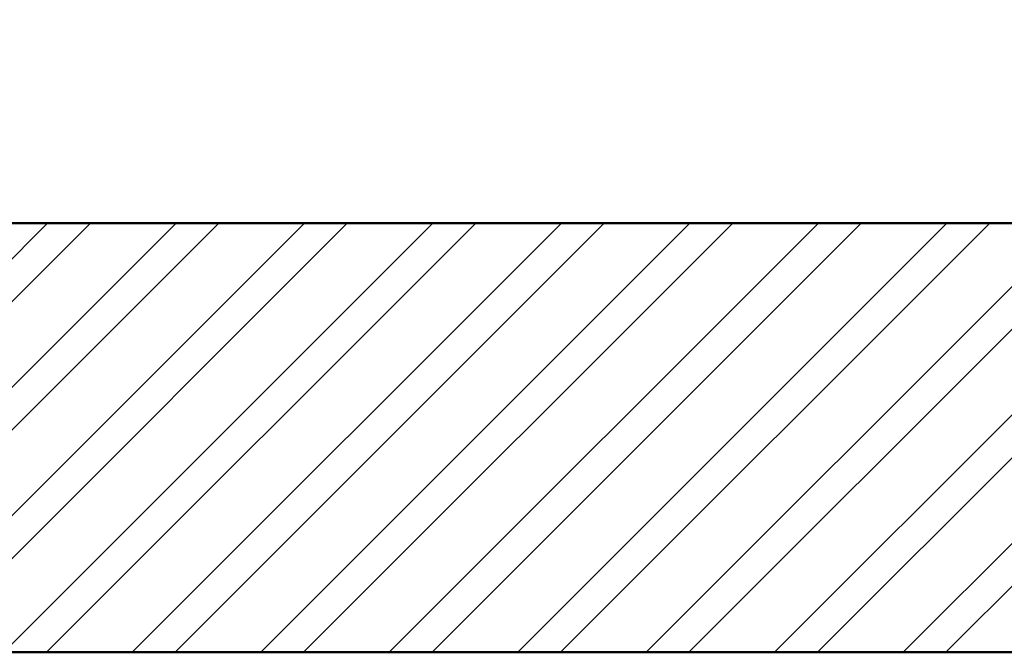
# Model space of a CAD drawing. Units: inches. Extents: x 3590 to 5167, y 65 to 1917.
# Tile 30 of 100: x 4947 to 4968, y 1326 to 1339. Entities that reach past the tile are written whole.
import ezdxf

# ---------------------------------------------------------------- set-up
doc = ezdxf.new("R2010")
doc.units = ezdxf.units.IN
for name, color, linetype, lineweight in [('A-FLOR-PATT', 8, 'Continuous', 13), ('A-WALL', 7, 'Continuous', 50), ('A-WALL-PATT', 251, 'Continuous', 13)]:
    doc.layers.add(name, color=color, linetype=linetype, lineweight=lineweight)

msp = doc.modelspace()

# ---------------------------------------------------------------- hatches: boundary and pattern name
at = {"layer": 'A-FLOR-PATT', "transparency": 33554687}
h = msp.add_hatch(dxfattribs=at)
h.set_pattern_fill('AR-HBONE', color=256, scale=0.2)
h.set_pattern_definition([(45, (-588.972, 0), (0, 28.73682), [60.96, -20.32]), (135, (-574.604, 14.368), (3e-15, 28.73682), [60.96, -20.32])])
h.paths.add_polyline_path([(5071.274, 1796.999), (4933.274, 1796.999), (4933.274, 1753.999), (4962.774, 1753.999, -0.414214), (4928.774, 1719.999), (4933.274, 1718.999), (4933.274, 1334.999), (5071.274, 1334.999)])
h.paths.add_polyline_path([(4951.78, 1521.077), (4951.715, 1521.04), (4951.563, 1520.895)], flags=16)
h.paths.add_polyline_path([(4952.267, 1521.376), (4952.198, 1521.371), (4952.198, 1521.356)], flags=0)
h.paths.add_polyline_path([(4967.051, 1529.728), (4965.231, 1528.694), (4963.411, 1527.714), (4961.756, 1526.851), (4963.589, 1527.449), (4964.036, 1527.478), (4962.975, 1527.249), (4961.76, 1526.852), (4959.792, 1525.834), (4958.005, 1524.895), (4956.24, 1523.93), (4954.504, 1522.919), (4954.129, 1522.682), (4953.361, 1521.997), (4953.366, 1521.998), (4953.605, 1522.064), (4955.106, 1522.761), (4956.921, 1523.434), (4958.678, 1523.915), (4960.358, 1524.2), (4961.945, 1524.286), (4964.171, 1524.108), (4965.958, 1523.309), (4963.863, 1522.976), (4965.187, 1522.499), (4963.366, 1522.497), (4961.545, 1522.487), (4959.764, 1522.461), (4958.304, 1522.419), (4957.974, 1522.388), (4956.307, 1522.232), (4954.718, 1522.071), (4953.251, 1521.899), (4953.525, 1521.623), (4954.331, 1521.379), (4956.243, 1521.23), (4958.039, 1520.93), (4959.684, 1520.483), (4961.16, 1519.896), (4963.107, 1518.8), (4964.393, 1517.325), (4962.973, 1517.726), (4964.558, 1516.661), (4965.407, 1515.708), (4963.507, 1516.322), (4961.68, 1517.005), (4959.935, 1517.745), (4958.282, 1518.528), (4956.732, 1519.343), (4955.295, 1520.175), (4954.672, 1520.572), (4954.513, 1520.627), (4955.658, 1519.318), (4956.703, 1517.982), (4957.644, 1516.647), (4958.485, 1515.334), (4959.55, 1513.524), (4960.438, 1511.769), (4958.841, 1513.62), (4957.452, 1515.325), (4955.819, 1517.459), (4956.665, 1515.448), (4957.111, 1513.923), (4957.447, 1511.714), (4957.076, 1509.793), (4956.538, 1511.11), (4955.992, 1512.569), (4955.444, 1514.125), (4954.898, 1515.735), (4954.357, 1517.356), (4953.824, 1518.943), (4953.305, 1520.452), (4953.065, 1521.116), (4952.971, 1521.146), (4952.949, 1521.086), (4952.73, 1520.199), (4953.37, 1518.024), (4953.757, 1516.373), (4954.051, 1514.765), (4954.264, 1513.221), (4954.471, 1511.131), (4954.497, 1510.402), (4954.409, 1511.76), (4954.264, 1513.221), (4954.051, 1514.765), (4953.757, 1516.373), (4953.37, 1518.024), (4952.877, 1519.698), (4952.716, 1520.141), (4952.533, 1519.059), (4952.374, 1517.789), (4952.219, 1516.312), (4952.046, 1514.6), (4951.833, 1512.626), (4951.557, 1510.363), (4951.203, 1512.168), (4950.852, 1514.339), (4950.985, 1516.376), (4951.66, 1518.286), (4952.593, 1520.481), (4952.357, 1521.13), (4951.855, 1520.328), (4950.839, 1518.908), (4949.777, 1517.587), (4948.916, 1516.617), (4948.111, 1515.256), (4947.089, 1513.554), (4945.889, 1511.615), (4946.326, 1513.402), (4946.562, 1514.249), (4945.528, 1513.327), (4944.581, 1512.531), (4946.018, 1514.508), (4947.204, 1516.048), (4947.893, 1517.313), (4949.307, 1518.764), (4950.414, 1519.767), (4950.451, 1519.806), (4952.267, 1521.376), (4951.645, 1521.493), (4950.404, 1521.18), (4948.044, 1520.359), (4946.119, 1519.452), (4944.572, 1518.475), (4943.35, 1517.443), (4941.997, 1515.92), (4941.661, 1515.275), (4942.813, 1516.99), (4944.572, 1518.475), (4946.119, 1519.452), (4948.044, 1520.359), (4950.404, 1521.18), (4951.645, 1521.493), (4949.647, 1521.868), (4948.6, 1521.756), (4947.126, 1521.57), (4945.42, 1521.348), (4943.45, 1521.105), (4941.183, 1520.856), (4942.86, 1521.613), (4943.873, 1522.03), (4942.952, 1521.909), (4941.41, 1521.485), (4939.543, 1520.67), (4938.968, 1520.226), (4940.733, 1521.299), (4942.952, 1521.909), (4943.702, 1522.008), (4945.894, 1522.7), (4947.565, 1522.714), (4948.921, 1522.566), (4951.131, 1522.183), (4950.971, 1522.297), (4948.129, 1523.006), (4946.035, 1523.707), (4944.232, 1524.521), (4942.707, 1525.461), (4941.444, 1526.537), (4940.43, 1527.761), (4939.649, 1529.143), (4941.421, 1528.122), (4943.147, 1527.132), (4944.841, 1526.175), (4946.514, 1525.25), (4948.179, 1524.359), (4948.365, 1524.263), (4946.475, 1526.045), (4945.181, 1527.54), (4944.19, 1529.033), (4943.496, 1530.54), (4943.278, 1531.36), (4942.498, 1531.919), (4943.114, 1531.762), (4942.959, 1533.659), (4944.14, 1531.989), (4944.612, 1531.323), (4946.202, 1530.463), (4947.486, 1529.509), (4948.79, 1528.226), (4950.368, 1526.237), (4949.485, 1528.155), (4948.851, 1530.123), (4948.491, 1532.041), (4948.381, 1533.918), (4948.501, 1535.76), (4948.827, 1537.573), (4949.418, 1535.565), (4949.957, 1533.569), (4950.464, 1531.586), (4950.961, 1529.617), (4951.391, 1527.954), (4951.724, 1530.687), (4952.201, 1532.58), (4952.889, 1534.33), (4953.77, 1535.951), (4954.827, 1537.46), (4954.521, 1535.39), (4954.273, 1533.937), (4955.58, 1535.663), (4956.748, 1536.739), (4956.159, 1534.78), (4955.589, 1532.873), (4955.043, 1531.006), (4954.525, 1529.166), (4954.038, 1527.341), (4953.638, 1525.733), (4953.611, 1525.586), (4953.398, 1524.166), (4953.382, 1524.009), (4954.07, 1525.476), (4954.912, 1527.022), (4956.136, 1528.894), (4957.847, 1530.577), (4959.376, 1531.54), (4958.256, 1530.104), (4957.143, 1528.663), (4956.066, 1527.243), (4955.056, 1525.871), (4954.141, 1524.571), (4953.352, 1523.372), (4953.311, 1523.303), (4953.273, 1522.925), (4953.261, 1522.382), (4954.103, 1523.373), (4954.63, 1524.284), (4955.961, 1526.358), (4957.23, 1528.13), (4958.421, 1529.609), (4960.037, 1531.368), (4961.374, 1532.375), (4962.101, 1532.77), (4961.07, 1531.061), (4959.987, 1529.438), (4958.869, 1527.908), (4958.15, 1527.007), (4959.803, 1528.003), (4961.589, 1528.793), (4963.391, 1529.328), (4965.211, 1529.632)], flags=16)
h.paths.add_polyline_path([(4962.944, 1523.182), (4961.107, 1523.422), (4960.392, 1523.362), (4962.35, 1523.331)], flags=0)
h.paths.add_polyline_path([(5049.541, 1584.551), (5049.476, 1584.515), (5049.325, 1584.37)], flags=16)
h.paths.add_polyline_path([(5050.028, 1584.851), (5049.959, 1584.845), (5049.959, 1584.83)], flags=0)
h.paths.add_polyline_path([(5042.333, 1581.949), (5043.88, 1582.926), (5045.806, 1583.833), (5048.165, 1584.654), (5049.406, 1584.967), (5047.408, 1585.342), (5046.361, 1585.231), (5044.888, 1585.044), (5043.181, 1584.822), (5041.211, 1584.579), (5038.944, 1584.33), (5040.622, 1585.087), (5041.634, 1585.504), (5040.713, 1585.383), (5039.171, 1584.959), (5037.304, 1584.144), (5036.729, 1583.7), (5038.494, 1584.773), (5040.713, 1585.383), (5041.463, 1585.482), (5043.655, 1586.174), (5045.326, 1586.188), (5046.682, 1586.04), (5048.893, 1585.657), (5048.732, 1585.771), (5045.891, 1586.48), (5043.796, 1587.181), (5041.994, 1587.996), (5040.468, 1588.935), (5039.205, 1590.011), (5038.191, 1591.235), (5037.41, 1592.617), (5039.182, 1591.596), (5040.909, 1590.607), (5042.602, 1589.649), (5044.275, 1588.724), (5045.94, 1587.833), (5046.126, 1587.738), (5044.237, 1589.519), (5042.942, 1591.015), (5041.952, 1592.508), (5041.257, 1594.014), (5041.039, 1594.834), (5040.26, 1595.393), (5040.875, 1595.237), (5040.721, 1597.133), (5041.901, 1595.463), (5042.373, 1594.798), (5043.963, 1593.938), (5045.247, 1592.983), (5046.552, 1591.701), (5048.129, 1589.712), (5047.247, 1591.63), (5046.613, 1593.597), (5046.252, 1595.515), (5046.142, 1597.392), (5046.262, 1599.234), (5046.588, 1601.047), (5047.179, 1599.039), (5047.718, 1597.043), (5048.225, 1595.06), (5048.722, 1593.091), (5049.152, 1591.429), (5049.485, 1594.161), (5049.962, 1596.054), (5050.65, 1597.804), (5051.532, 1599.425), (5052.589, 1600.934), (5052.283, 1598.864), (5052.034, 1597.411), (5053.341, 1599.137), (5054.509, 1600.213), (5053.92, 1598.254), (5053.35, 1596.348), (5052.805, 1594.48), (5052.286, 1592.64), (5051.799, 1590.815), (5051.4, 1589.207), (5051.373, 1589.06), (5051.159, 1587.64), (5051.143, 1587.483), (5051.831, 1588.95), (5052.673, 1590.496), (5053.898, 1592.368), (5055.608, 1594.051), (5057.137, 1595.014), (5056.017, 1593.578), (5054.904, 1592.137), (5053.828, 1590.717), (5052.817, 1589.345), (5051.902, 1588.046), (5051.113, 1586.846), (5051.072, 1586.777), (5051.034, 1586.399), (5051.022, 1585.856), (5051.864, 1586.847), (5052.391, 1587.758), (5053.723, 1589.832), (5054.991, 1591.604), (5056.182, 1593.083), (5057.798, 1594.842), (5059.135, 1595.849), (5059.863, 1596.244), (5058.831, 1594.535), (5057.749, 1592.912), (5056.63, 1591.382), (5055.912, 1590.482), (5057.564, 1591.477), (5059.35, 1592.267), (5061.152, 1592.802), (5062.972, 1593.106), (5064.812, 1593.203), (5062.992, 1592.169), (5061.172, 1591.188), (5059.518, 1590.325), (5061.35, 1590.924), (5061.797, 1590.952), (5060.737, 1590.723), (5059.521, 1590.326), (5057.553, 1589.308), (5055.766, 1588.369), (5054.002, 1587.404), (5052.265, 1586.393), (5051.891, 1586.156), (5051.122, 1585.471), (5051.127, 1585.472), (5051.366, 1585.538), (5052.867, 1586.235), (5054.682, 1586.908), (5056.439, 1587.389), (5058.12, 1587.675), (5059.706, 1587.76), (5061.933, 1587.583), (5063.719, 1586.783), (5061.624, 1586.45), (5062.949, 1585.973), (5061.127, 1585.971), (5059.307, 1585.961), (5057.525, 1585.935), (5056.065, 1585.893), (5055.735, 1585.862), (5054.068, 1585.707), (5052.479, 1585.546), (5051.012, 1585.373), (5051.286, 1585.097), (5052.092, 1584.853), (5054.004, 1584.704), (5055.8, 1584.404), (5057.446, 1583.958), (5058.921, 1583.37), (5060.868, 1582.274), (5062.154, 1580.799), (5060.734, 1581.2), (5062.32, 1580.135), (5063.168, 1579.182), (5061.269, 1579.796), (5059.441, 1580.479), (5057.696, 1581.219), (5056.043, 1582.003), (5054.493, 1582.817), (5053.057, 1583.649), (5052.433, 1584.047), (5052.274, 1584.101), (5053.42, 1582.793), (5054.464, 1581.457), (5055.405, 1580.121), (5056.247, 1578.809), (5057.311, 1576.998), (5058.199, 1575.244), (5056.602, 1577.094), (5055.213, 1578.799), (5053.58, 1580.933), (5054.427, 1578.922), (5054.872, 1577.397), (5055.208, 1575.189), (5054.838, 1573.267), (5054.299, 1574.584), (5053.754, 1576.043), (5053.206, 1577.599), (5052.659, 1579.209), (5052.118, 1580.83), (5051.585, 1582.417), (5051.066, 1583.927), (5050.826, 1584.59), (5050.733, 1584.62), (5050.711, 1584.561), (5050.491, 1583.673), (5051.131, 1581.498), (5051.518, 1579.847), (5051.813, 1578.24), (5052.026, 1576.695), (5052.233, 1574.605), (5052.258, 1573.876), (5052.17, 1575.234), (5052.026, 1576.695), (5051.813, 1578.24), (5051.518, 1579.847), (5051.131, 1581.498), (5050.638, 1583.172), (5050.477, 1583.615), (5050.294, 1582.533), (5050.136, 1581.263), (5049.981, 1579.786), (5049.807, 1578.074), (5049.594, 1576.1), (5049.318, 1573.837), (5048.965, 1575.642), (5048.613, 1577.813), (5048.747, 1579.85), (5049.421, 1581.76), (5050.354, 1583.955), (5050.118, 1584.604), (5049.616, 1583.802), (5048.6, 1582.382), (5047.538, 1581.061), (5046.677, 1580.091), (5045.872, 1578.73), (5044.85, 1577.028), (5043.651, 1575.089), (5044.087, 1576.877), (5044.324, 1577.723), (5043.289, 1576.801), (5042.342, 1576.005), (5043.779, 1577.982), (5044.966, 1579.522), (5045.655, 1580.787), (5047.068, 1582.239), (5048.175, 1583.241), (5048.213, 1583.28), (5050.028, 1584.851), (5049.406, 1584.967), (5048.165, 1584.654), (5045.806, 1583.833), (5043.88, 1582.926), (5042.333, 1581.949), (5041.111, 1580.917), (5039.758, 1579.394), (5039.423, 1578.749), (5040.575, 1580.464)], flags=16)
h.paths.add_polyline_path([(4954.799, 1533.12), (4954.262, 1532.079), (4953.831, 1530.935), (4953.505, 1529.636), (4953.283, 1528.133), (4953.167, 1526.376), (4953.156, 1524.315), (4953.277, 1521.236), (4952.802, 1521.842), (4951.557, 1521.998), (4950.976, 1521.961), (4952.661, 1521.941), (4952.802, 1521.842), (4953.152, 1523.593), (4953.167, 1526.376), (4953.283, 1528.133), (4953.609, 1530.346), (4954.456, 1532.592)], flags=0)
h.paths.add_polyline_path([(5050.563, 1585.316), (5049.318, 1585.472), (5048.737, 1585.435), (5050.422, 1585.415), (5050.563, 1585.316), (5050.914, 1587.067), (5050.928, 1589.851), (5051.045, 1591.607), (5051.371, 1593.82), (5052.217, 1596.066), (5052.56, 1596.594), (5052.024, 1595.554), (5051.592, 1594.409), (5051.266, 1593.11), (5051.045, 1591.607), (5050.928, 1589.851), (5050.918, 1587.789), (5051.038, 1584.71)], flags=0)
h.paths.add_polyline_path([(5058.153, 1586.836), (5060.111, 1586.805), (5060.705, 1586.656), (5058.868, 1586.896)], flags=0)
h.paths.add_polyline_path([(5049.541, 1430.936), (5049.476, 1430.9), (5049.325, 1430.755)], flags=16)
h.paths.add_polyline_path([(5050.028, 1431.236), (5049.959, 1431.231), (5049.959, 1431.215)], flags=0)
h.paths.add_polyline_path([(5046.588, 1447.432), (5047.179, 1445.425), (5047.718, 1443.429), (5048.225, 1441.446), (5048.722, 1439.476), (5049.152, 1437.814), (5049.485, 1440.546), (5049.962, 1442.439), (5050.65, 1444.189), (5051.532, 1445.811), (5052.589, 1447.319), (5052.283, 1445.249), (5052.034, 1443.796), (5053.341, 1445.522), (5054.509, 1446.598), (5053.92, 1444.64), (5053.35, 1442.733), (5052.805, 1440.865), (5052.286, 1439.025), (5051.799, 1437.201), (5051.4, 1435.592), (5051.373, 1435.445), (5051.159, 1434.025), (5051.143, 1433.868), (5051.831, 1435.335), (5052.673, 1436.881), (5053.898, 1438.753), (5055.608, 1440.436), (5057.137, 1441.4), (5056.017, 1439.963), (5054.904, 1438.522), (5053.828, 1437.102), (5052.817, 1435.73), (5051.902, 1434.431), (5051.113, 1433.231), (5051.072, 1433.162), (5051.034, 1432.784), (5051.022, 1432.242), (5051.864, 1433.232), (5052.391, 1434.143), (5053.723, 1436.217), (5054.991, 1437.989), (5056.182, 1439.468), (5057.798, 1441.227), (5059.135, 1442.235), (5059.863, 1442.629), (5058.831, 1440.921), (5057.749, 1439.298), (5056.63, 1437.767), (5055.912, 1436.867), (5057.564, 1437.863), (5059.35, 1438.652), (5061.152, 1439.187), (5062.972, 1439.491), (5064.812, 1439.588), (5062.992, 1438.554), (5061.172, 1437.573), (5059.518, 1436.71), (5061.35, 1437.309), (5061.797, 1437.337), (5060.737, 1437.108), (5059.521, 1436.711), (5057.553, 1435.693), (5055.766, 1434.754), (5054.002, 1433.789), (5052.265, 1432.778), (5051.891, 1432.541), (5051.122, 1431.856), (5051.127, 1431.857), (5051.366, 1431.923), (5052.867, 1432.62), (5054.682, 1433.293), (5056.439, 1433.775), (5058.12, 1434.06), (5059.706, 1434.145), (5061.933, 1433.968), (5063.719, 1433.168), (5061.624, 1432.835), (5062.949, 1432.358), (5061.127, 1432.357), (5059.307, 1432.346), (5057.525, 1432.32), (5056.065, 1432.278), (5055.735, 1432.248), (5054.068, 1432.092), (5052.479, 1431.931), (5051.012, 1431.759), (5051.286, 1431.482), (5052.092, 1431.238), (5054.004, 1431.089), (5055.8, 1430.789), (5057.446, 1430.343), (5058.921, 1429.755), (5060.868, 1428.66), (5062.154, 1427.185), (5060.734, 1427.585), (5062.32, 1426.52), (5063.168, 1425.567), (5061.269, 1426.181), (5059.441, 1426.865), (5057.696, 1427.604), (5056.043, 1428.388), (5054.493, 1429.202), (5053.057, 1430.034), (5052.433, 1430.432), (5052.274, 1430.487), (5053.42, 1429.178), (5054.464, 1427.842), (5055.405, 1426.506), (5056.247, 1425.194), (5057.311, 1423.383), (5058.199, 1421.629), (5056.602, 1423.479), (5055.213, 1425.184), (5053.58, 1427.318), (5054.427, 1425.307), (5054.872, 1423.782), (5055.208, 1421.574), (5054.838, 1419.652), (5054.299, 1420.97), (5053.754, 1422.428), (5053.206, 1423.984), (5052.659, 1425.595), (5052.118, 1427.215), (5051.585, 1428.802), (5051.066, 1430.312), (5050.826, 1430.975), (5050.733, 1431.005), (5050.711, 1430.946), (5050.491, 1430.058), (5051.131, 1427.883), (5051.518, 1426.232), (5051.813, 1424.625), (5052.026, 1423.081), (5052.233, 1420.991), (5052.258, 1420.261), (5052.17, 1421.619), (5052.026, 1423.081), (5051.813, 1424.625), (5051.518, 1426.232), (5051.131, 1427.883), (5050.638, 1429.558), (5050.477, 1430.001), (5050.294, 1428.918), (5050.136, 1427.648), (5049.981, 1426.171), (5049.807, 1424.459), (5049.594, 1422.485), (5049.318, 1420.222), (5048.965, 1422.028), (5048.613, 1424.199), (5048.747, 1426.235), (5049.421, 1428.146), (5050.354, 1430.34), (5050.118, 1430.989), (5049.616, 1430.187), (5048.6, 1428.768), (5047.538, 1427.446), (5046.677, 1426.477), (5045.872, 1425.116), (5044.85, 1423.413), (5043.651, 1421.474), (5044.087, 1423.262), (5044.324, 1424.109), (5043.289, 1423.186), (5042.342, 1422.391), (5043.779, 1424.368), (5044.966, 1425.907), (5045.655, 1427.173), (5047.068, 1428.624), (5048.175, 1429.627), (5048.213, 1429.666), (5050.028, 1431.236), (5049.406, 1431.353), (5048.165, 1431.039), (5045.806, 1430.218), (5043.88, 1429.311), (5042.333, 1428.334), (5041.111, 1427.302), (5039.758, 1425.779), (5039.423, 1425.134), (5040.575, 1426.849), (5042.333, 1428.334), (5043.88, 1429.311), (5045.806, 1430.218), (5048.165, 1431.039), (5049.406, 1431.353), (5047.408, 1431.727), (5046.361, 1431.616), (5044.888, 1431.429), (5043.181, 1431.207), (5041.211, 1430.964), (5038.944, 1430.715), (5040.622, 1431.472), (5041.634, 1431.89), (5040.713, 1431.769), (5039.171, 1431.345), (5037.304, 1430.53), (5036.729, 1430.085), (5038.494, 1431.158), (5040.713, 1431.769), (5041.463, 1431.867), (5043.655, 1432.559), (5045.326, 1432.573), (5046.682, 1432.425), (5048.893, 1432.042), (5048.732, 1432.156), (5045.891, 1432.865), (5043.796, 1433.566), (5041.994, 1434.381), (5040.468, 1435.321), (5039.205, 1436.396), (5038.191, 1437.62), (5037.41, 1439.002), (5039.182, 1437.982), (5040.909, 1436.992), (5042.602, 1436.034), (5044.275, 1435.109), (5045.94, 1434.218), (5046.126, 1434.123), (5044.237, 1435.904), (5042.942, 1437.4), (5041.952, 1438.893), (5041.257, 1440.399), (5041.039, 1441.219), (5040.26, 1441.778), (5040.875, 1441.622), (5040.721, 1443.518), (5041.901, 1441.848), (5042.373, 1441.183), (5043.963, 1440.323), (5045.247, 1439.369), (5046.552, 1438.086), (5048.129, 1436.097), (5047.247, 1438.015), (5046.613, 1439.982), (5046.252, 1441.901), (5046.142, 1443.778), (5046.262, 1445.619)], flags=16)
h.paths.add_polyline_path([(5052.382, 1444.255), (5051.623, 1442.78), (5052.024, 1441.939), (5052.56, 1442.98)], flags=0)
h.paths.add_polyline_path([(5050.563, 1431.701), (5049.318, 1431.857), (5048.737, 1431.821), (5050.422, 1431.8)], flags=0)
h.paths.add_polyline_path([(5058.153, 1433.221), (5060.111, 1433.19), (5060.705, 1433.041), (5058.868, 1433.281)], flags=0)
h.paths.add_polyline_path([(5049.541, 1352.285), (5049.476, 1352.249), (5049.325, 1352.104)], flags=16)
h.paths.add_polyline_path([(5050.028, 1352.585), (5049.959, 1352.58), (5049.959, 1352.564)], flags=0)
h.paths.add_polyline_path([(5046.588, 1368.781), (5047.179, 1366.774), (5047.718, 1364.778), (5048.225, 1362.795), (5048.722, 1360.825), (5049.152, 1359.163), (5049.485, 1361.896), (5049.962, 1363.789), (5050.65, 1365.538), (5051.532, 1367.16), (5052.589, 1368.669), (5052.283, 1366.598), (5052.034, 1365.145), (5053.341, 1366.871), (5054.509, 1367.947), (5053.92, 1365.989), (5053.35, 1364.082), (5052.805, 1362.214), (5052.286, 1360.374), (5051.799, 1358.55), (5051.4, 1356.942), (5051.373, 1356.794), (5051.159, 1355.374), (5051.143, 1355.218), (5051.831, 1356.684), (5052.673, 1358.23), (5053.898, 1360.102), (5055.608, 1361.786), (5057.137, 1362.749), (5056.017, 1361.313), (5054.904, 1359.872), (5053.828, 1358.452), (5052.817, 1357.079), (5051.902, 1355.78), (5051.113, 1354.581), (5051.072, 1354.512), (5051.034, 1354.133), (5051.022, 1353.591), (5051.864, 1354.581), (5052.391, 1355.492), (5053.723, 1357.566), (5054.991, 1359.338), (5056.182, 1360.817), (5057.798, 1362.577), (5059.135, 1363.584), (5059.863, 1363.979), (5058.831, 1362.27), (5057.749, 1360.647), (5056.63, 1359.117), (5055.912, 1358.216), (5057.564, 1359.212), (5059.35, 1360.001), (5061.152, 1360.536), (5062.972, 1360.841), (5064.812, 1360.937), (5062.992, 1359.903), (5061.172, 1358.923), (5059.518, 1358.059), (5061.35, 1358.658), (5061.797, 1358.687), (5060.737, 1358.458), (5059.521, 1358.061), (5057.553, 1357.043), (5055.766, 1356.103), (5054.002, 1355.138), (5052.265, 1354.127), (5051.891, 1353.89), (5051.122, 1353.206), (5051.127, 1353.206), (5051.366, 1353.272), (5052.867, 1353.969), (5054.682, 1354.643), (5056.439, 1355.124), (5058.12, 1355.409), (5059.706, 1355.495), (5061.933, 1355.317), (5063.719, 1354.518), (5061.624, 1354.184), (5062.949, 1353.708), (5061.127, 1353.706), (5059.307, 1353.695), (5057.525, 1353.669), (5056.065, 1353.627), (5055.735, 1353.597), (5054.068, 1353.441), (5052.479, 1353.28), (5051.012, 1353.108), (5051.286, 1352.831), (5052.092, 1352.587), (5054.004, 1352.439), (5055.8, 1352.138), (5057.446, 1351.692), (5058.921, 1351.104), (5060.868, 1350.009), (5062.154, 1348.534), (5060.734, 1348.935), (5062.32, 1347.869), (5063.168, 1346.916), (5061.269, 1347.53), (5059.441, 1348.214), (5057.696, 1348.954), (5056.043, 1349.737), (5054.493, 1350.551), (5053.057, 1351.383), (5052.433, 1351.781), (5052.274, 1351.836), (5053.42, 1350.527), (5054.464, 1349.191), (5055.405, 1347.855), (5056.247, 1346.543), (5057.311, 1344.733), (5058.199, 1342.978), (5056.602, 1344.828), (5055.213, 1346.534), (5053.58, 1348.667), (5054.427, 1346.656), (5054.872, 1345.132), (5055.208, 1342.923), (5054.838, 1341.002), (5054.299, 1342.319), (5053.754, 1343.778), (5053.206, 1345.334), (5052.659, 1346.944), (5052.118, 1348.564), (5051.585, 1350.151), (5051.066, 1351.661), (5050.826, 1352.324), (5050.733, 1352.355), (5050.711, 1352.295), (5050.491, 1351.408), (5051.131, 1349.232), (5051.518, 1347.581), (5051.813, 1345.974), (5052.026, 1344.43), (5052.233, 1342.34), (5052.258, 1341.61), (5052.17, 1342.969), (5052.026, 1344.43), (5051.813, 1345.974), (5051.518, 1347.581), (5051.131, 1349.232), (5050.638, 1350.907), (5050.477, 1351.35), (5050.294, 1350.267), (5050.136, 1348.997), (5049.981, 1347.52), (5049.807, 1345.809), (5049.594, 1343.835), (5049.318, 1341.571), (5048.965, 1343.377), (5048.613, 1345.548), (5048.747, 1347.585), (5049.421, 1349.495), (5050.354, 1351.689), (5050.118, 1352.339), (5049.616, 1351.536), (5048.6, 1350.117), (5047.538, 1348.795), (5046.677, 1347.826), (5045.872, 1346.465), (5044.85, 1344.763), (5043.651, 1342.824), (5044.087, 1344.611), (5044.324, 1345.458), (5043.289, 1344.535), (5042.342, 1343.74), (5043.779, 1345.717), (5044.966, 1347.256), (5045.655, 1348.522), (5047.068, 1349.973), (5048.175, 1350.976), (5048.213, 1351.015), (5050.028, 1352.585), (5049.406, 1352.702), (5048.165, 1352.388), (5045.806, 1351.567), (5043.88, 1350.661), (5042.333, 1349.683), (5041.111, 1348.651), (5039.758, 1347.128), (5039.423, 1346.483), (5040.575, 1348.198), (5042.333, 1349.683), (5043.88, 1350.661), (5045.806, 1351.567), (5048.165, 1352.388), (5049.406, 1352.702), (5047.408, 1353.076), (5046.361, 1352.965), (5044.888, 1352.779), (5043.181, 1352.556), (5041.211, 1352.313), (5038.944, 1352.065), (5040.622, 1352.821), (5041.634, 1353.239), (5040.713, 1353.118), (5039.171, 1352.694), (5037.304, 1351.879), (5036.729, 1351.434), (5038.494, 1352.508), (5040.713, 1353.118), (5041.463, 1353.216), (5043.655, 1353.909), (5045.326, 1353.923), (5046.682, 1353.774), (5048.893, 1353.391), (5048.732, 1353.506), (5045.891, 1354.214), (5043.796, 1354.915), (5041.994, 1355.73), (5040.468, 1356.67), (5039.205, 1357.746), (5038.191, 1358.969), (5037.41, 1360.352), (5039.182, 1359.331), (5040.909, 1358.341), (5042.602, 1357.383), (5044.275, 1356.458), (5045.94, 1355.567), (5046.126, 1355.472), (5044.237, 1357.253), (5042.942, 1358.749), (5041.952, 1360.242), (5041.257, 1361.748), (5041.039, 1362.568), (5040.26, 1363.128), (5040.875, 1362.971), (5040.721, 1364.867), (5041.901, 1363.197), (5042.373, 1362.532), (5043.963, 1361.672), (5045.247, 1360.718), (5046.552, 1359.435), (5048.129, 1357.446), (5047.247, 1359.364), (5046.613, 1361.331), (5046.252, 1363.25), (5046.142, 1365.127), (5046.262, 1366.969)], flags=16)
h.paths.add_polyline_path([(5052.382, 1365.604), (5051.623, 1364.129), (5052.024, 1363.288), (5052.56, 1364.329)], flags=0)
h.paths.add_polyline_path([(4951.78, 1698.041), (4951.715, 1698.005), (4951.563, 1697.859)], flags=16)
h.paths.add_polyline_path([(4952.267, 1698.341), (4952.198, 1698.335), (4952.198, 1698.32)], flags=0)
h.paths.add_polyline_path([(4957.076, 1686.757), (4956.538, 1688.074), (4955.992, 1689.533), (4955.444, 1691.089), (4954.898, 1692.699), (4954.357, 1694.32), (4953.824, 1695.907), (4953.305, 1697.417), (4953.065, 1698.08), (4952.971, 1698.11), (4952.949, 1698.051), (4952.73, 1697.163), (4953.37, 1694.988), (4953.757, 1693.337), (4954.051, 1691.729), (4954.264, 1690.185), (4954.471, 1688.095), (4954.497, 1687.366), (4954.409, 1688.724), (4954.264, 1690.185), (4954.051, 1691.729), (4953.757, 1693.337), (4953.37, 1694.988), (4952.877, 1696.662), (4952.716, 1697.105), (4952.533, 1696.023), (4952.374, 1694.753), (4952.219, 1693.276), (4952.046, 1691.564), (4951.833, 1689.59), (4951.557, 1687.327), (4951.203, 1689.132), (4950.852, 1691.303), (4950.985, 1693.34), (4951.66, 1695.25), (4952.593, 1697.445), (4952.357, 1698.094), (4951.855, 1697.292), (4950.839, 1695.872), (4949.777, 1694.551), (4948.916, 1693.581), (4948.111, 1692.22), (4947.089, 1690.518), (4945.889, 1688.579), (4946.326, 1690.366), (4946.562, 1691.213), (4945.528, 1690.291), (4944.581, 1689.495), (4946.018, 1691.472), (4947.204, 1693.012), (4947.893, 1694.277), (4949.307, 1695.729), (4950.414, 1696.731), (4950.451, 1696.77), (4952.267, 1698.341), (4951.645, 1698.457), (4950.404, 1698.144), (4948.044, 1697.323), (4946.119, 1696.416), (4944.572, 1695.439), (4943.35, 1694.407), (4941.997, 1692.884), (4941.661, 1692.239), (4942.813, 1693.954), (4944.572, 1695.439), (4946.119, 1696.416), (4948.044, 1697.323), (4950.404, 1698.144), (4951.645, 1698.457), (4949.647, 1698.832), (4948.6, 1698.72), (4947.126, 1698.534), (4945.42, 1698.312), (4943.45, 1698.069), (4941.183, 1697.82), (4942.86, 1698.577), (4943.873, 1698.994), (4942.952, 1698.873), (4941.41, 1698.449), (4939.543, 1697.634), (4938.968, 1697.19), (4940.733, 1698.263), (4942.952, 1698.873), (4943.702, 1698.972), (4945.894, 1699.664), (4947.565, 1699.678), (4948.921, 1699.53), (4951.131, 1699.147), (4950.971, 1699.261), (4948.129, 1699.97), (4946.035, 1700.671), (4944.232, 1701.486), (4942.707, 1702.425), (4941.444, 1703.501), (4940.43, 1704.725), (4939.649, 1706.107), (4941.421, 1705.086), (4943.147, 1704.097), (4944.841, 1703.139), (4946.514, 1702.214), (4948.179, 1701.323), (4948.365, 1701.227), (4946.475, 1703.009), (4945.181, 1704.505), (4944.19, 1705.997), (4943.496, 1707.504), (4943.278, 1708.324), (4942.498, 1708.883), (4943.114, 1708.727), (4942.959, 1710.623), (4944.14, 1708.953), (4944.612, 1708.287), (4946.202, 1707.428), (4947.486, 1706.473), (4948.79, 1705.191), (4950.368, 1703.202), (4949.485, 1705.12), (4948.851, 1707.087), (4948.491, 1709.005), (4948.381, 1710.882), (4948.501, 1712.724), (4948.827, 1714.537), (4949.418, 1712.529), (4949.957, 1710.533), (4950.464, 1708.55), (4950.961, 1706.581), (4951.391, 1704.919), (4951.724, 1707.651), (4952.201, 1709.544), (4952.889, 1711.294), (4953.77, 1712.915), (4954.827, 1714.424), (4954.521, 1712.354), (4954.273, 1710.901), (4955.58, 1712.627), (4956.748, 1713.703), (4956.159, 1711.744), (4955.589, 1709.837), (4955.043, 1707.97), (4954.525, 1706.13), (4954.038, 1704.305), (4953.638, 1702.697), (4953.611, 1702.55), (4953.398, 1701.13), (4953.382, 1700.973), (4954.07, 1702.44), (4954.912, 1703.986), (4956.136, 1705.858), (4957.847, 1707.541), (4959.376, 1708.504), (4958.256, 1707.068), (4957.143, 1705.627), (4956.066, 1704.207), (4955.056, 1702.835), (4954.141, 1701.536), (4953.352, 1700.336), (4953.311, 1700.267), (4953.273, 1699.889), (4953.261, 1699.346), (4954.103, 1700.337), (4954.63, 1701.248), (4955.961, 1703.322), (4957.23, 1705.094), (4958.421, 1706.573), (4960.037, 1708.332), (4961.374, 1709.339), (4962.101, 1709.734), (4961.07, 1708.025), (4959.987, 1706.402), (4958.869, 1704.872), (4958.15, 1703.972), (4959.803, 1704.967), (4961.589, 1705.757), (4963.391, 1706.292), (4965.211, 1706.596), (4967.051, 1706.692), (4965.231, 1705.659), (4963.411, 1704.678), (4961.756, 1703.815), (4963.589, 1704.413), (4964.036, 1704.442), (4962.975, 1704.213), (4961.76, 1703.816), (4959.792, 1702.798), (4958.005, 1701.859), (4956.24, 1700.894), (4954.504, 1699.883), (4954.129, 1699.646), (4953.361, 1698.961), (4953.366, 1698.962), (4953.605, 1699.028), (4955.106, 1699.725), (4956.921, 1700.398), (4958.678, 1700.879), (4960.358, 1701.164), (4961.945, 1701.25), (4964.171, 1701.073), (4965.958, 1700.273), (4963.863, 1699.94), (4965.187, 1699.463), (4963.366, 1699.461), (4961.545, 1699.451), (4959.764, 1699.425), (4958.304, 1699.383), (4957.974, 1699.352), (4956.307, 1699.197), (4954.718, 1699.036), (4953.251, 1698.863), (4953.525, 1698.587), (4954.331, 1698.343), (4956.243, 1698.194), (4958.039, 1697.894), (4959.684, 1697.447), (4961.16, 1696.86), (4963.107, 1695.764), (4964.393, 1694.289), (4962.973, 1694.69), (4964.558, 1693.625), (4965.407, 1692.672), (4963.507, 1693.286), (4961.68, 1693.969), (4959.935, 1694.709), (4958.282, 1695.492), (4956.732, 1696.307), (4955.295, 1697.139), (4954.672, 1697.536), (4954.513, 1697.591), (4955.658, 1696.282), (4956.703, 1694.946), (4957.644, 1693.611), (4958.485, 1692.298), (4959.55, 1690.488), (4960.438, 1688.733), (4958.841, 1690.584), (4957.452, 1692.289), (4955.819, 1694.423), (4956.665, 1692.412), (4957.111, 1690.887), (4957.447, 1688.678)], flags=16)
h.paths.add_polyline_path([(5050.563, 1353.05), (5049.318, 1353.207), (5048.737, 1353.17), (5050.422, 1353.15)], flags=0)
h.paths.add_polyline_path([(4951.78, 1351.486), (4951.715, 1351.45), (4951.563, 1351.305)], flags=16)
h.paths.add_polyline_path([(4952.267, 1351.786), (4952.198, 1351.78), (4952.198, 1351.765)], flags=0)
h.paths.add_polyline_path([(4954.827, 1367.869), (4954.521, 1365.799), (4954.273, 1364.346), (4955.58, 1366.072), (4956.748, 1367.148), (4956.159, 1365.19), (4955.589, 1363.283), (4955.043, 1361.415), (4954.525, 1359.575), (4954.038, 1357.751), (4953.638, 1356.142), (4953.611, 1355.995), (4953.398, 1354.575), (4953.382, 1354.418), (4954.07, 1355.885), (4954.912, 1357.431), (4956.136, 1359.303), (4957.847, 1360.986), (4959.376, 1361.95), (4958.256, 1360.513), (4957.143, 1359.072), (4956.066, 1357.652), (4955.056, 1356.28), (4954.141, 1354.981), (4953.352, 1353.781), (4953.311, 1353.712), (4953.273, 1353.334), (4953.261, 1352.792), (4954.103, 1353.782), (4954.63, 1354.693), (4955.961, 1356.767), (4957.23, 1358.539), (4958.421, 1360.018), (4960.037, 1361.777), (4961.374, 1362.785), (4962.101, 1363.179), (4961.07, 1361.471), (4959.987, 1359.848), (4958.869, 1358.317), (4958.15, 1357.417), (4959.803, 1358.413), (4961.589, 1359.202), (4963.391, 1359.737), (4965.211, 1360.041), (4967.051, 1360.138), (4965.231, 1359.104), (4963.411, 1358.123), (4961.756, 1357.26), (4963.589, 1357.859), (4964.036, 1357.887), (4962.975, 1357.658), (4961.76, 1357.261), (4959.792, 1356.243), (4958.005, 1355.304), (4956.24, 1354.339), (4954.504, 1353.328), (4954.129, 1353.091), (4953.361, 1352.406), (4953.366, 1352.407), (4953.605, 1352.473), (4955.106, 1353.17), (4956.921, 1353.843), (4958.678, 1354.325), (4960.358, 1354.61), (4961.945, 1354.695), (4964.171, 1354.518), (4965.958, 1353.718), (4963.863, 1353.385), (4965.187, 1352.908), (4963.366, 1352.907), (4961.545, 1352.896), (4959.764, 1352.87), (4958.304, 1352.828), (4957.974, 1352.798), (4956.307, 1352.642), (4954.718, 1352.481), (4953.251, 1352.309), (4953.525, 1352.032), (4954.331, 1351.788), (4956.243, 1351.639), (4958.039, 1351.339), (4959.684, 1350.893), (4961.16, 1350.305), (4963.107, 1349.21), (4964.393, 1347.735), (4962.973, 1348.135), (4964.558, 1347.07), (4965.407, 1346.117), (4963.507, 1346.731), (4961.68, 1347.414), (4959.935, 1348.154), (4958.282, 1348.938), (4956.732, 1349.752), (4955.295, 1350.584), (4954.672, 1350.982), (4954.513, 1351.036), (4955.658, 1349.728), (4956.703, 1348.392), (4957.644, 1347.056), (4958.485, 1345.744), (4959.55, 1343.933), (4960.438, 1342.179), (4958.841, 1344.029), (4957.452, 1345.734), (4955.819, 1347.868), (4956.665, 1345.857), (4957.111, 1344.332), (4957.447, 1342.124), (4957.076, 1340.202), (4956.538, 1341.52), (4955.992, 1342.978), (4955.444, 1344.534), (4954.898, 1346.145), (4954.357, 1347.765), (4953.824, 1349.352), (4953.305, 1350.862), (4953.065, 1351.525), (4952.971, 1351.555), (4952.949, 1351.496), (4952.73, 1350.608), (4953.37, 1348.433), (4953.757, 1346.782), (4954.051, 1345.175), (4954.264, 1343.631), (4954.471, 1341.541), (4954.497, 1340.811), (4954.409, 1342.169), (4954.264, 1343.631), (4954.051, 1345.175), (4953.757, 1346.782), (4953.37, 1348.433), (4952.877, 1350.108), (4952.716, 1350.551), (4952.533, 1349.468), (4952.374, 1348.198), (4952.219, 1346.721), (4952.046, 1345.009), (4951.833, 1343.035), (4951.557, 1340.772), (4951.203, 1342.578), (4950.852, 1344.749), (4950.985, 1346.785), (4951.66, 1348.696), (4952.593, 1350.89), (4952.357, 1351.539), (4951.855, 1350.737), (4950.839, 1349.318), (4949.777, 1347.996), (4948.916, 1347.027), (4948.111, 1345.665), (4947.089, 1343.963), (4945.889, 1342.024), (4946.326, 1343.812), (4946.562, 1344.659), (4945.528, 1343.736), (4944.581, 1342.941), (4946.018, 1344.918), (4947.204, 1346.457), (4947.893, 1347.723), (4949.307, 1349.174), (4950.414, 1350.177), (4950.451, 1350.216), (4952.267, 1351.786), (4951.645, 1351.903), (4950.404, 1351.589), (4948.044, 1350.768), (4946.119, 1349.861), (4944.572, 1348.884), (4943.35, 1347.852), (4941.997, 1346.329), (4941.661, 1345.684), (4942.813, 1347.399), (4944.572, 1348.884), (4946.119, 1349.861), (4948.044, 1350.768), (4950.404, 1351.589), (4951.645, 1351.903), (4949.647, 1352.277), (4948.6, 1352.166), (4947.126, 1351.979), (4945.42, 1351.757), (4943.45, 1351.514), (4941.183, 1351.265), (4942.86, 1352.022), (4943.873, 1352.44), (4942.952, 1352.319), (4941.41, 1351.895), (4939.543, 1351.08), (4938.968, 1350.635), (4940.733, 1351.708), (4942.952, 1352.319), (4943.702, 1352.417), (4945.894, 1353.109), (4947.565, 1353.123), (4948.921, 1352.975), (4951.131, 1352.592), (4950.971, 1352.706), (4948.129, 1353.415), (4946.035, 1354.116), (4944.232, 1354.931), (4942.707, 1355.871), (4941.444, 1356.946), (4940.43, 1358.17), (4939.649, 1359.552), (4941.421, 1358.532), (4943.147, 1357.542), (4944.841, 1356.584), (4946.514, 1355.659), (4948.179, 1354.768), (4948.365, 1354.673), (4946.475, 1356.454), (4945.181, 1357.95), (4944.19, 1359.443), (4943.496, 1360.949), (4943.278, 1361.769), (4942.498, 1362.328), (4943.114, 1362.172), (4942.959, 1364.068), (4944.14, 1362.398), (4944.612, 1361.733), (4946.202, 1360.873), (4947.486, 1359.919), (4948.79, 1358.636), (4950.368, 1356.647), (4949.485, 1358.565), (4948.851, 1360.532), (4948.491, 1362.451), (4948.381, 1364.328), (4948.501, 1366.169), (4948.827, 1367.982), (4949.418, 1365.975), (4949.957, 1363.979), (4950.464, 1361.995), (4950.961, 1360.026), (4951.391, 1358.364), (4951.724, 1361.096), (4952.201, 1362.989), (4952.889, 1364.739), (4953.77, 1366.361)], flags=16)
h.paths.add_polyline_path([(4954.799, 1363.53), (4954.262, 1362.489), (4953.831, 1361.344), (4953.505, 1360.045), (4953.283, 1358.543), (4953.167, 1356.786), (4953.156, 1354.724), (4953.277, 1351.646), (4952.802, 1352.251), (4951.557, 1352.407), (4950.976, 1352.371), (4952.661, 1352.35), (4952.802, 1352.251), (4953.152, 1354.002), (4953.167, 1356.786), (4953.283, 1358.543), (4953.609, 1360.755), (4954.456, 1363.001)], flags=0)
h.paths.add_polyline_path([(4952.802, 1698.806), (4951.557, 1698.962), (4950.976, 1698.925), (4952.661, 1698.905), (4952.802, 1698.806), (4953.152, 1700.557), (4953.167, 1703.34), (4953.283, 1705.097), (4953.609, 1707.31), (4954.456, 1709.556), (4954.799, 1710.084), (4954.262, 1709.043), (4953.831, 1707.899), (4953.505, 1706.6), (4953.283, 1705.097), (4953.167, 1703.34), (4953.156, 1701.279), (4953.277, 1698.2)], flags=0)
h.paths.add_polyline_path([(4962.944, 1700.146), (4961.107, 1700.386), (4960.392, 1700.326), (4962.35, 1700.295)], flags=0)
h.paths.add_polyline_path([(5058.153, 1354.57), (5060.111, 1354.539), (5060.705, 1354.391), (5058.868, 1354.631)], flags=0)
h.paths.add_polyline_path([(4962.944, 1353.591), (4961.107, 1353.831), (4960.392, 1353.771), (4962.35, 1353.74)], flags=0)
h.paths.add_polyline_path([(5049.541, 1778.72), (5049.476, 1778.684), (5049.325, 1778.539)], flags=16)
h.paths.add_polyline_path([(5050.028, 1779.02), (5049.959, 1779.014), (5049.959, 1778.999)], flags=0)
h.paths.add_polyline_path([(5052.258, 1768.045), (5052.17, 1769.403), (5052.026, 1770.864), (5051.813, 1772.409), (5051.518, 1774.016), (5051.131, 1775.667), (5050.638, 1777.341), (5050.477, 1777.784), (5050.294, 1776.702), (5050.136, 1775.432), (5049.981, 1773.955), (5049.807, 1772.243), (5049.594, 1770.269), (5049.318, 1768.006), (5048.965, 1769.811), (5048.613, 1771.982), (5048.747, 1774.019), (5049.421, 1775.929), (5050.354, 1778.124), (5050.118, 1778.773), (5049.616, 1777.971), (5048.6, 1776.551), (5047.538, 1775.23), (5046.677, 1774.26), (5045.872, 1772.899), (5044.85, 1771.197), (5043.651, 1769.258), (5044.087, 1771.046), (5044.324, 1771.892), (5043.289, 1770.97), (5042.342, 1770.174), (5043.779, 1772.151), (5044.966, 1773.691), (5045.655, 1774.956), (5047.068, 1776.408), (5048.175, 1777.41), (5048.213, 1777.449), (5050.028, 1779.02), (5049.406, 1779.136), (5048.165, 1778.823), (5045.806, 1778.002), (5043.88, 1777.095), (5042.333, 1776.118), (5041.111, 1775.086), (5039.758, 1773.563), (5039.423, 1772.918), (5040.575, 1774.633), (5042.333, 1776.118), (5043.88, 1777.095), (5045.806, 1778.002), (5048.165, 1778.823), (5049.406, 1779.136), (5047.408, 1779.511), (5046.361, 1779.4), (5044.888, 1779.213), (5043.181, 1778.991), (5041.211, 1778.748), (5038.944, 1778.499), (5040.622, 1779.256), (5041.634, 1779.673), (5040.713, 1779.552), (5039.171, 1779.128), (5037.304, 1778.313), (5036.729, 1777.869), (5038.494, 1778.942), (5040.713, 1779.552), (5041.463, 1779.651), (5043.655, 1780.343), (5045.326, 1780.357), (5046.682, 1780.209), (5048.893, 1779.826), (5048.732, 1779.94), (5045.891, 1780.649), (5043.796, 1781.35), (5041.994, 1782.165), (5040.468, 1783.104), (5039.205, 1784.18), (5038.191, 1785.404), (5037.41, 1786.786), (5039.182, 1785.765), (5040.909, 1784.776), (5042.602, 1783.818), (5044.275, 1782.893), (5045.94, 1782.002), (5046.126, 1781.907), (5044.237, 1783.688), (5042.942, 1785.184), (5041.952, 1786.677), (5041.257, 1788.183), (5041.039, 1789.003), (5040.26, 1789.562), (5040.875, 1789.406), (5040.721, 1791.302), (5041.901, 1789.632), (5042.373, 1788.967), (5043.963, 1788.107), (5045.247, 1787.152), (5046.552, 1785.87), (5048.129, 1783.881), (5047.247, 1785.799), (5046.613, 1787.766), (5046.252, 1789.684), (5046.142, 1791.561), (5046.262, 1793.403), (5046.588, 1795.216), (5047.179, 1793.208), (5047.718, 1791.213), (5048.225, 1789.229), (5048.722, 1787.26), (5049.152, 1785.598), (5049.485, 1788.33), (5049.962, 1790.223), (5050.65, 1791.973), (5051.532, 1793.594), (5052.589, 1795.103), (5052.283, 1793.033), (5052.034, 1791.58), (5053.341, 1793.306), (5054.509, 1794.382), (5053.92, 1792.423), (5053.35, 1790.517), (5052.805, 1788.649), (5052.286, 1786.809), (5051.799, 1784.984), (5051.4, 1783.376), (5051.373, 1783.229), (5051.159, 1781.809), (5051.143, 1781.652), (5051.831, 1783.119), (5052.673, 1784.665), (5053.898, 1786.537), (5055.608, 1788.22), (5057.137, 1789.183), (5056.017, 1787.747), (5054.904, 1786.306), (5053.828, 1784.886), (5052.817, 1783.514), (5051.902, 1782.215), (5051.113, 1781.015), (5051.072, 1780.946), (5051.034, 1780.568), (5051.022, 1780.025), (5051.864, 1781.016), (5052.391, 1781.927), (5053.723, 1784.001), (5054.991, 1785.773), (5056.182, 1787.252), (5057.798, 1789.011), (5059.135, 1790.018), (5059.863, 1790.413), (5058.831, 1788.704), (5057.749, 1787.081), (5056.63, 1785.551), (5055.912, 1784.651), (5057.564, 1785.646), (5059.35, 1786.436), (5061.152, 1786.971), (5062.972, 1787.275), (5064.812, 1787.372), (5062.992, 1786.338), (5061.172, 1785.357), (5059.518, 1784.494), (5061.35, 1785.093), (5061.797, 1785.121), (5060.737, 1784.892), (5059.521, 1784.495), (5057.553, 1783.477), (5055.766, 1782.538), (5054.002, 1781.573), (5052.265, 1780.562), (5051.891, 1780.325), (5051.122, 1779.64), (5051.127, 1779.641), (5051.366, 1779.707), (5052.867, 1780.404), (5054.682, 1781.077), (5056.439, 1781.558), (5058.12, 1781.844), (5059.706, 1781.929), (5061.933, 1781.752), (5063.719, 1780.952), (5061.624, 1780.619), (5062.949, 1780.142), (5061.127, 1780.14), (5059.307, 1780.13), (5057.525, 1780.104), (5056.065, 1780.062), (5055.735, 1780.031), (5054.068, 1779.876), (5052.479, 1779.715), (5051.012, 1779.542), (5051.286, 1779.266), (5052.092, 1779.022), (5054.004, 1778.873), (5055.8, 1778.573), (5057.446, 1778.127), (5058.921, 1777.539), (5060.868, 1776.443), (5062.154, 1774.968), (5060.734, 1775.369), (5062.32, 1774.304), (5063.168, 1773.351), (5061.269, 1773.965), (5059.441, 1774.648), (5057.696, 1775.388), (5056.043, 1776.172), (5054.493, 1776.986), (5053.057, 1777.818), (5052.433, 1778.216), (5052.274, 1778.27), (5053.42, 1776.962), (5054.464, 1775.626), (5055.405, 1774.29), (5056.247, 1772.978), (5057.311, 1771.167), (5058.199, 1769.413), (5056.602, 1771.263), (5055.213, 1772.968), (5053.58, 1775.102), (5054.427, 1773.091), (5054.872, 1771.566), (5055.208, 1769.358), (5054.838, 1767.436), (5054.299, 1768.753), (5053.754, 1770.212), (5053.206, 1771.768), (5052.659, 1773.378), (5052.118, 1774.999), (5051.585, 1776.586), (5051.066, 1778.096), (5050.826, 1778.759), (5050.733, 1778.789), (5050.711, 1778.73), (5050.491, 1777.842), (5051.131, 1775.667), (5051.518, 1774.016), (5051.813, 1772.409), (5052.026, 1770.864), (5052.233, 1768.774)], flags=16)
h.paths.add_polyline_path([(5050.563, 1779.485), (5049.318, 1779.641), (5048.737, 1779.604), (5050.422, 1779.584), (5050.563, 1779.485), (5050.914, 1781.236), (5050.928, 1784.02), (5051.045, 1785.776), (5051.371, 1787.989), (5052.217, 1790.235), (5052.56, 1790.763), (5052.024, 1789.723), (5051.592, 1788.578), (5051.266, 1787.279), (5051.045, 1785.776), (5050.928, 1784.02), (5050.918, 1781.958), (5051.038, 1778.879)], flags=0)
h.paths.add_polyline_path([(5058.153, 1781.005), (5060.111, 1780.974), (5060.705, 1780.825), (5058.868, 1781.065)], flags=0)
at = {"layer": 'A-WALL-PATT', "transparency": 33554687}
h = msp.add_hatch(dxfattribs=at)
h.set_pattern_fill('ANSI32', color=256, scale=0.2)
h.paths.add_polyline_path([(4684.274, 1805.999), (4591.274, 1805.999), (4591.274, 1796.999), (4639.274, 1796.999), (4639.274, 1790.999), (4648.274, 1790.999), (4648.274, 1796.999), (4684.274, 1796.999)])
h.paths.add_polyline_path([(4543.274, 1805.999), (4420.274, 1805.999), (4420.274, 1784.999), (4429.274, 1784.999), (4429.274, 1796.999), (4445.919, 1796.999), (4543.274, 1796.999)])
h.paths.add_polyline_path([(4828.274, 1805.999), (4744.274, 1805.999), (4744.274, 1796.999), (4828.274, 1796.999)])
h.paths.add_polyline_path([(4648.274, 1754.999), (4639.274, 1754.999), (4639.274, 1655.999), (4546.274, 1655.999), (4546.274, 1649.999), (4549.274, 1649.999), (4549.274, 1553.999), (4429.274, 1553.999), (4429.274, 1583.999), (4420.274, 1583.999), (4420.274, 1538.999), (4429.274, 1538.999), (4429.274, 1544.999), (4639.274, 1544.999), (4639.274, 1538.999), (4648.274, 1538.999), (4648.274, 1559.999), (4639.274, 1559.999), (4639.274, 1553.999), (4555.274, 1553.999), (4555.274, 1649.999), (4639.274, 1649.999), (4639.274, 1589.999), (4648.274, 1589.999)])
h.paths.add_polyline_path([(4516.274, 1655.999), (4429.274, 1655.999), (4429.274, 1736.999), (4420.274, 1736.999), (4420.274, 1619.999), (4429.274, 1619.999), (4429.274, 1649.999), (4516.274, 1649.999)], flags=17)
h.paths.add_polyline_path([(5080.274, 1805.999), (4888.274, 1805.999), (4888.274, 1796.999), (4924.274, 1796.999), (4924.274, 1754.999), (4933.274, 1754.999), (4933.274, 1796.999), (5071.274, 1796.999), (5071.274, 1334.999), (4933.274, 1334.999), (4933.274, 1565.999), (4924.274, 1565.999), (4924.274, 1334.999), (4898.774, 1334.999), (4898.774, 1325.999), (5080.274, 1325.999)])
h.paths.add_polyline_path([(4933.274, 1718.999), (4924.274, 1718.999), (4924.274, 1637.999), (4933.274, 1637.999)], flags=17)
h.paths.add_polyline_path([(4802.774, 1334.999), (4777.274, 1334.999), (4777.274, 1502.999), (4756.274, 1502.999), (4756.274, 1493.999), (4768.274, 1493.999), (4768.274, 1430.999), (4696.274, 1430.999), (4696.274, 1493.999), (4708.274, 1493.999), (4708.274, 1502.999), (4639.274, 1502.999), (4639.274, 1493.999), (4687.274, 1493.999), (4687.274, 1430.999), (4681.274, 1430.999), (4681.274, 1421.999), (4768.274, 1421.999), (4768.274, 1334.999), (4726.274, 1334.999), (4726.274, 1325.999), (4802.774, 1325.999)])
h.paths.add_polyline_path([(4690.274, 1334.999), (4648.274, 1334.999), (4648.274, 1352.867), (4648.274, 1421.999), (4651.274, 1421.999), (4651.274, 1430.999), (4639.274, 1430.999), (4639.274, 1334.999), (4633.274, 1334.999), (4633.274, 1325.999), (4690.274, 1325.999)])
h.paths.add_polyline_path([(4585.274, 1334.999), (4584.724, 1334.999), (4429.274, 1334.999), (4429.274, 1490.999), (4420.274, 1490.999), (4420.274, 1325.999), (4585.274, 1325.999)])

# ---------------------------------------------------------------- linework, layer by layer
at = {"layer": 'A-WALL'}
msp.add_line((5071.274, 1334.999), (4933.274, 1334.999), dxfattribs=at)
msp.add_lwpolyline([(5080.274, 1805.999), (5080.274, 1325.999), (4420.274, 1325.999), (4420.274, 1805.999)], close=True, dxfattribs=at)

doc.saveas('drawing.dxf')
